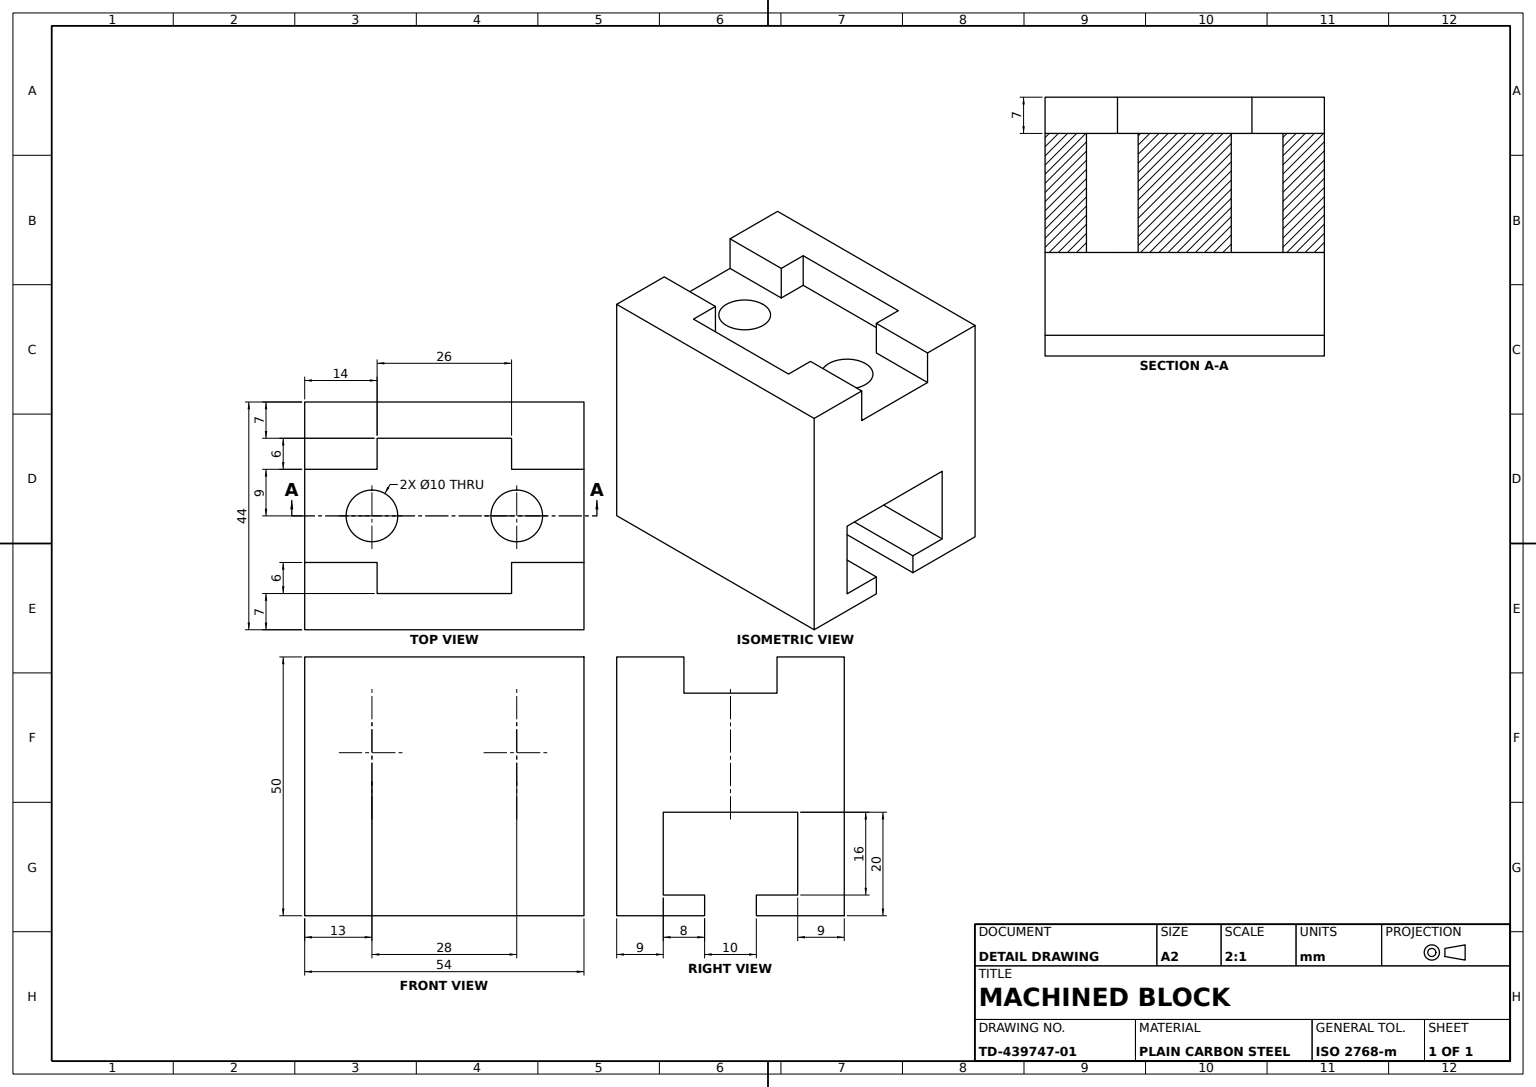
from build123d import *

# Parameters (mm, degrees)
BASE_BLOCK_SKETCH_W       = 54
BASE_BLOCK_SKETCH_H       = 50
BASE_BLOCK_54X50X44_DEPTH = 44
TOP_POCKET_7_DEEP_DEPTH   = 7
T_SLOT_CUT_DEPTH          = 75.006756448
POCKET_HOLES_SKETCH_R     = 5
POCKET_HOLES_2X_10_DEPTH  = 68.186308129


with BuildPart() as part:
    # Base Block Sketch → Base Block 54x50x44 (new body)
    with BuildSketch(Plane.XY):
        Rectangle(BASE_BLOCK_SKETCH_W, BASE_BLOCK_SKETCH_H)
    extrude(amount=-BASE_BLOCK_54X50X44_DEPTH)

    # Top Pocket Sketch → Top Pocket 7 Deep (cut)
    with BuildSketch(Plane(origin=(0, 25, 0), x_dir=(1, 0, 0), z_dir=(0, 1, 0))):
        Polygon((-13, 37), (13, 37), (13, 31), (27, 31), (27, 13), (13, 13), (13, 7), (-13, 7), (-13, 13), (-27, 13), (-27, 31), (-13, 31), align=None)
    extrude(amount=-TOP_POCKET_7_DEEP_DEPTH, mode=Mode.SUBTRACT)

    # T-Slot Sketch → T-Slot Cut (cut, through all)
    with BuildSketch(Plane.ZY.offset(27)):
        Polygon((-27, -25), (-27, -21), (-35, -21), (-35, -5), (-9, -5), (-9, -21), (-17, -21), (-17, -25), align=None)
    extrude(amount=-T_SLOT_CUT_DEPTH, mode=Mode.SUBTRACT)

    # Pocket Holes Sketch → Pocket Holes 2xØ10 (cut, through all)
    with BuildSketch(Plane(origin=(0, 18, 0), x_dir=(1, 0, 0), z_dir=(0, 1, 0))):
        with Locations(Location((-14, 22, 0), (0, 0, 270))):
            Circle(POCKET_HOLES_SKETCH_R)
        with Locations(Location((14, 22, 0), (0, 0, 270))):
            Circle(POCKET_HOLES_SKETCH_R)
    extrude(amount=-POCKET_HOLES_2X_10_DEPTH, mode=Mode.SUBTRACT)


solid = part.part
